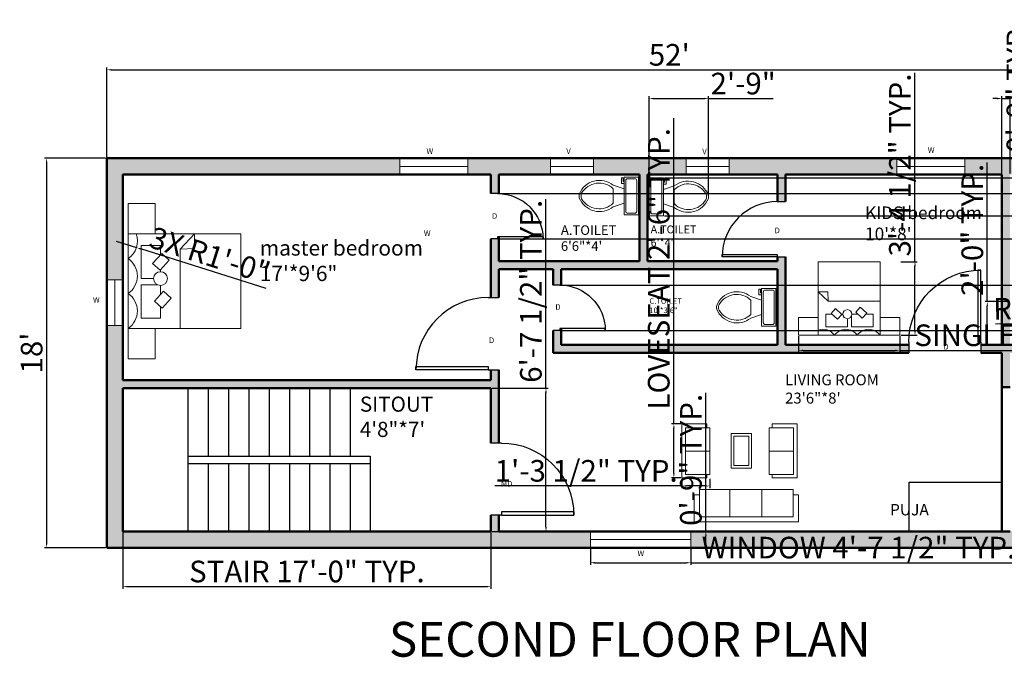
# Model space of a CAD drawing. Units: inches. Extents: x 2225 to 3094, y 1739 to 2599.
# Tile 1 of 5: x 2234 to 2780, y 1739 to 2092. Entities that reach past the tile are written whole.
import ezdxf

# ---------------------------------------------------------------- set-up
doc = ezdxf.new("R2010")
doc.units = ezdxf.units.IN
for name, color, linetype, lineweight in [('A-ANNO-DIMS', 2, 'Continuous', 18), ('A-ANNO-TEXT', 7, 'Continuous', 18), ('A-ANNO-TITL', 7, 'Continuous', 35), ('A-AREA-IDEN', 7, 'Continuous', 18), ('A-DOOR', 4, 'Continuous', 25), ('A-FLOR-CASE', 9, 'Continuous', 25), ('A-FLOR-FIXT', 9, 'Continuous', 18), ('A-FLOR-STRS', 7, 'Continuous', 25), ('A-FURN', 8, 'Continuous', 18), ('A-WALL-PATT', 160, 'Continuous', 13), ('WALL', 7, 'Continuous', 50), ('WINDOW', 130, 'Continuous', 18)]:
    doc.layers.add(name, color=color, linetype=linetype, lineweight=lineweight)
doc.styles.get("Standard").update_dxf_attribs({"font": 'arial.ttf'})
doc.dimstyles.new('ISO-25', dxfattribs={"dimtxt": 12, "dimasz": 2.5, "dimexe": 1.25, "dimexo": 0.625, "dimtad": 1, "dimdec": 0, "dimlunit": 4, "dimtxsty": 'Standard', "dimcen": 2.5, "dimadec": 0, "dimazin": 0, "dimtfac": 1, "dimtdec": 0, "dimtmove": 0, "dimatfit": 3, "dimfxl": 1, "dimarcsym": 0})

# ---------------------------------------------------------------- blocks, each defined once
blk = doc.blocks.new('*U2')
for p, q in [((9.5, -6), (9.5, -2)), ((-10, -8.5), (-8, -8.5)), ((-10, -9.5), (-10, -8.5)), ((-7, -9.5), (-10, -9.5)), ((-8, -8.5), (-8, -8)), ((-7, -8), (-7, -9.5)), ((-4, -8), (-6, -14)), ((4, -8), (6, -14)), ((4, -14), (-4, -14))]:
    blk.add_line(p, q)
blk.add_lwpolyline([(10.5, -8), (10.5, 0), (-10.5, 0), (-10.5, -8)], close=True)
for points in [[(-9.5, -2), (-9.5, -6)], [(8.5, -1), (-8.5, -1)], [(-8.5, -7), (8.5, -7)]]:
    blk.add_lwpolyline(points)
for centre, radius, start, end in [((-8.62, -1.88), 0.884, 81.8699, 188.1301), ((8.62, -1.88), 0.884, 351.8699, 98.1301), ((-8.62, -6.12), 0.884, 171.8699, 278.1301), ((8.62, -6.12), 0.884, 261.8699, 8.1301), ((3.52, -21.58), 12.17, 141.4691, 247.9714), ((4.2, -21.82), 11.33, 136.3677, 238.9468), ((-3.52, -21.58), 12.17, 292.0284, 38.5307), ((-4.2, -21.82), 11.33, 301.053, 43.6321), ((0, -27.88), 4, 245.7318, 294.2682), ((0, -29), 4, 254.8605, 285.1395)]:
    blk.add_arc(centre, radius, start, end)
blk = doc.blocks.new('*U4')
for p, q in [((0, 0), (0, -6)), ((40, 0), (40, -6))]:
    blk.add_line(p, q)
blk.add_lwpolyline([(0, 0), (0, 40), (1.75, 40), (1.75, 0)], close=True)
blk.add_arc((0, 0), 40, 0, 90)
blk = doc.blocks.new('*D7')
at = {"layer": 'A-ANNO-DIMS', "color": 0, "lineweight": -2, "transparency": 16777216}
for p, q in [((2282.56, 2016.04), (2282.56, 2065.75)), ((2285.06, 2064.5), (2904.06, 2064.5)), ((2906.56, 2016.04), (2906.56, 2065.75))]:
    blk.add_line(p, q, dxfattribs=at)
at = {"layer": 'A-ANNO-DIMS', "color": 0, "transparency": 16777216}
for points in [[(2285.06, 2064.92), (2285.06, 2064.08), (2282.56, 2064.5)], [(2904.06, 2064.92), (2904.06, 2064.08), (2906.56, 2064.5)]]:
    blk.add_solid(points, dxfattribs=at)
at = {"layer": 'Defpoints', "color": 0, "transparency": 16777216}
for p in [(2906.56, 2064.5), (2282.56, 2015.41), (2906.56, 2015.41)]:
    blk.add_point(p, dxfattribs=at)
at = {"layer": 'A-ANNO-DIMS', "color": 0, "transparency": 16777216, "insert": (2594.56, 2071.25), "char_height": 12, "attachment_point": 5}
blk.add_mtext("52'", dxfattribs=at)
blk = doc.blocks.new('*D8')
at = {"layer": 'A-ANNO-DIMS', "color": 0, "lineweight": -2, "transparency": 16777216}
for p, q in [((2281.93, 2015.41), (2247.95, 2015.41)), ((2249.2, 2012.91), (2249.2, 1801.91)), ((2281.93, 1799.41), (2247.95, 1799.41))]:
    blk.add_line(p, q, dxfattribs=at)
at = {"layer": 'A-ANNO-DIMS', "color": 0, "transparency": 16777216}
for points in [[(2248.78, 2012.91), (2249.61, 2012.91), (2249.2, 2015.41)], [(2248.78, 1801.91), (2249.61, 1801.91), (2249.2, 1799.41)]]:
    blk.add_solid(points, dxfattribs=at)
at = {"layer": 'Defpoints', "color": 0, "transparency": 16777216}
for p in [(2282.56, 2015.41), (2249.2, 1799.41), (2282.56, 1799.41)]:
    blk.add_point(p, dxfattribs=at)
at = {"layer": 'A-ANNO-DIMS', "color": 0, "transparency": 16777216, "insert": (2242.45, 1907.41), "char_height": 12, "attachment_point": 5, "rotation": 90}
blk.add_mtext("18'", dxfattribs=at)
blk = doc.blocks.new('STAIR-RETURN')
for p, q in [((0, 79.5), (36, 79.5)), ((36, 79.5), (36, 0)), ((47.27, 79.5), (47.27, 41.75)), ((58.52, 79.5), (58.52, 41.75)), ((69.77, 79.5), (69.77, 41.75)), ((81.01, 79.5), (81.01, 41.75)), ((92.26, 79.5), (92.26, 41.75)), ((103.51, 79.5), (103.51, 41.75)), ((114.75, 79.5), (114.75, 41.75)), ((204, 79.5), (126, 79.5)), ((126, 79.5), (126, 41.75)), ((36, 41.75), (126, 41.75)), ((126, 41.75), (137, 41.75)), ((137, 41.75), (137, 0)), ((36, 37.75), (126, 37.75)), ((47.27, 37.75), (47.27, 0)), ((58.52, 37.75), (58.52, 0)), ((69.77, 37.75), (69.77, 0)), ((81.01, 37.75), (81.01, 0)), ((92.26, 37.75), (92.26, 0)), ((103.51, 37.75), (103.51, 0)), ((114.75, 37.75), (114.75, 0)), ((126, 37.75), (137, 37.75)), ((126, 37.75), (126, 0))]:
    blk.add_line(p, q)
blk = doc.blocks.new('BED-MASTER')
for p, q in [((28.8, 60.76), (36.78, 69.23)), ((36.78, 69.23), (36.78, 61.09)), ((36.78, 61.09), (28.8, 60.76)), ((28.8, 16.79), (28.8, 60.76))]:
    blk.add_line(p, q)
for points in [[(0, 69.23), (14.9, 69.23), (14.9, 86.02), (0, 86.02)], [(0, 16.79), (62.39, 16.79), (62.39, 69.23), (0, 69.23)], [(13.53, 52.86), (18.54, 58.39), (22.68, 54.63), (17.67, 49.11)], [(14.58, 31.86), (19.59, 37.39), (23.73, 33.63), (18.72, 28.11)], [(0, 0), (14.9, 0), (14.9, 16.79), (0, 16.79)]]:
    blk.add_lwpolyline(points, close=True)
for points in [[(17.87, 57.65), (17.87, 62.86), (7.1, 62.86), (7.1, 44.44), (14.04, 44.44)], [(17.87, 48.27), (17.87, 49.33)], [(16.36, 40.92), (7.1, 40.92), (7.1, 22.51), (17.87, 22.51), (17.87, 28.87)], [(17.87, 35.5), (17.87, 40.61)]]:
    blk.add_lwpolyline(points)
blk.add_circle((17.87, 44.44), 3.83)
for centre, end in [((-6.76, 65.2), 19.9878), ((-6.76, 45.83), 55.0719), ((-6.76, 26.47), 55.0719)]:
    blk.add_arc(centre, 11.81, 304.9281, end)
blk = doc.blocks.new('BED-SINGLE')
for p, q in [((16.5, 18.81), (10.96, 24.02)), ((10.96, 24.02), (16.28, 24.02)), ((16.28, 24.02), (16.5, 18.81)), ((45.21, 18.81), (16.5, 18.81))]:
    blk.add_line(p, q)
for points in [[(45.21, 0), (45.21, 40.75), (10.96, 40.75), (10.96, 0)], [(21.65, 8.84), (18.05, 12.11), (20.5, 14.81), (24.1, 11.54)], [(35.37, 9.52), (31.76, 12.79), (34.21, 15.49), (37.82, 12.22)], [(10.96, 0), (10.96, 9.73), (0, 9.73), (0, 0)], [(56.18, 0), (56.18, 9.73), (45.21, 9.73), (45.21, 0)]]:
    blk.add_lwpolyline(points, close=True)
for points in [[(18.53, 11.67), (15.12, 11.67), (15.12, 4.64), (27.15, 4.64), (27.15, 9.17)], [(24.65, 11.67), (23.96, 11.67)], [(29.45, 10.68), (29.45, 4.64), (41.48, 4.64), (41.48, 11.67), (37.32, 11.67)], [(32.99, 11.67), (29.65, 11.67)]]:
    blk.add_lwpolyline(points)
blk.add_circle((27.15, 11.67), 2.5)
for centre, end in [((13.6, -4.42), 109.9878), ((26.25, -4.42), 145.0719), ((38.89, -4.42), 145.0719)]:
    blk.add_arc(centre, 7.71, 34.9281, end)
blk = doc.blocks.new('SOFA-THREE-SEAT')
for p, q in [((19.92, 17.92), (19.92, 2.75)), ((37.66, 17.92), (37.66, 2.75)), ((3.02, 14.97), (0, 14.97)), ((0, 14.97), (0, 0)), ((57.91, 14.97), (54.99, 14.97)), ((57.91, 0), (57.91, 14.97)), ((0, 0), (57.91, 0))]:
    blk.add_line(p, q)
blk.add_lwpolyline([(3.02, 2.75), (54.99, 2.75), (54.99, 17.92), (3.02, 17.92)], close=True)
blk = doc.blocks.new('SOFA-TWO-SEAT')
for p, q in [((1.66, 27.74), (1.66, 29.95)), ((1.66, 29.95), (15.43, 29.95)), ((15.43, 29.95), (15.43, 0)), ((0, 14.84), (13.39, 14.84)), ((1.66, 0), (1.66, 1.94)), ((15.43, 0), (1.66, 0))]:
    blk.add_line(p, q)
blk.add_lwpolyline([(13.39, 1.94), (0, 1.94), (0, 27.74), (13.39, 27.74)], close=True)
blk = doc.blocks.new('TABLE-COFFEE')
for points in [[(0, 0), (11.17, 0), (11.17, 19.11), (0, 19.11)], [(1.5, 1.5), (9.67, 1.5), (9.67, 17.61), (1.5, 17.61)]]:
    blk.add_lwpolyline(points, close=True)
blk = doc.blocks.new('WIN-55P7IN')
blk.add_line((0, 4.5), (55.68, 4.5))
blk.add_lwpolyline([(0, 0), (55.68, 0), (55.68, 9), (0, 9)], close=True)
blk = doc.blocks.new('*D26')
at = {"layer": 'A-ANNO-DIMS', "color": 0, "lineweight": -2, "transparency": 16777216}
for p, q in [((2666.23, 1916.66), (2666.23, 1907.61)), ((2722.41, 1916.66), (2722.41, 1907.61)), ((2668.73, 1908.86), (2719.91, 1908.86)), ((2722.41, 1908.86), (2904.52, 1908.86))]:
    blk.add_line(p, q, dxfattribs=at)
at = {"layer": 'A-ANNO-DIMS', "color": 0, "transparency": 16777216}
for points in [[(2668.73, 1909.27), (2668.73, 1908.44), (2666.23, 1908.86)], [(2719.91, 1909.27), (2719.91, 1908.44), (2722.41, 1908.86)]]:
    blk.add_solid(points, dxfattribs=at)
at = {"layer": 'Defpoints', "color": 0, "transparency": 16777216}
for p in [(2666.23, 1917.28), (2722.41, 1917.28), (2722.41, 1908.86)]:
    blk.add_point(p, dxfattribs=at)
at = {"layer": 'A-ANNO-DIMS', "color": 0, "transparency": 16777216, "insert": (2814.71, 1915.69), "char_height": 12, "attachment_point": 5}
blk.add_mtext('SINGLE BED 4\'-8" TYP.', dxfattribs=at)
blk = doc.blocks.new('*D27')
at = {"layer": 'A-ANNO-DIMS', "color": 0, "lineweight": -2, "transparency": 16777216}
for p, q in [((2730.83, 1958.03), (2730.83, 2062.88)), ((2723.03, 1958.03), (2732.08, 1958.03)), ((2730.83, 1919.78), (2730.83, 1955.53)), ((2723.03, 1917.28), (2732.08, 1917.28))]:
    blk.add_line(p, q, dxfattribs=at)
at = {"layer": 'A-ANNO-DIMS', "color": 0, "transparency": 16777216}
for points in [[(2730.42, 1955.53), (2731.25, 1955.53), (2730.83, 1958.03)], [(2730.42, 1919.78), (2731.25, 1919.78), (2730.83, 1917.28)]]:
    blk.add_solid(points, dxfattribs=at)
at = {"layer": 'Defpoints', "color": 0, "transparency": 16777216}
for p in [(2722.41, 1958.03), (2730.83, 1958.03), (2722.41, 1917.28)]:
    blk.add_point(p, dxfattribs=at)
at = {"layer": 'A-ANNO-DIMS', "color": 0, "transparency": 16777216, "insert": (2724, 2011.7), "char_height": 12, "attachment_point": 5, "rotation": 90}
blk.add_mtext('3\'-4 1/2" TYP.', dxfattribs=at)
blk = doc.blocks.new('*D34')
at = {"layer": 'A-ANNO-DIMS', "color": 0, "lineweight": -2, "transparency": 16777216}
for p, q in [((2597.09, 1868.1), (2597.09, 2037.63)), ((2600.96, 1868.1), (2595.84, 1868.1)), ((2597.09, 1840.65), (2597.09, 1865.6)), ((2600.96, 1838.15), (2595.84, 1838.15))]:
    blk.add_line(p, q, dxfattribs=at)
at = {"layer": 'A-ANNO-DIMS', "color": 0, "transparency": 16777216}
for points in [[(2596.67, 1865.6), (2597.51, 1865.6), (2597.09, 1868.1)], [(2596.67, 1840.65), (2597.51, 1840.65), (2597.09, 1838.15)]]:
    blk.add_solid(points, dxfattribs=at)
at = {"layer": 'Defpoints', "color": 0, "transparency": 16777216}
for p in [(2597.09, 1868.1), (2601.58, 1868.1), (2601.58, 1838.15)]:
    blk.add_point(p, dxfattribs=at)
at = {"layer": 'A-ANNO-DIMS', "color": 0, "transparency": 16777216, "insert": (2590.26, 1954.11), "char_height": 12, "attachment_point": 5, "rotation": 90}
blk.add_mtext('LOVESEAT 2\'-6" TYP.', dxfattribs=at)
blk = doc.blocks.new('*D35')
at = {"layer": 'A-ANNO-DIMS', "color": 0, "lineweight": -2, "transparency": 16777216}
for p, q in [((2601.58, 1837.52), (2601.58, 1832.41)), ((2617.01, 1837.52), (2617.01, 1832.41)), ((2601.58, 1833.66), (2497.86, 1833.66)), ((2614.51, 1833.66), (2604.08, 1833.66))]:
    blk.add_line(p, q, dxfattribs=at)
at = {"layer": 'A-ANNO-DIMS', "color": 0, "transparency": 16777216}
for points in [[(2604.08, 1834.07), (2604.08, 1833.24), (2601.58, 1833.66)], [(2614.51, 1834.07), (2614.51, 1833.24), (2617.01, 1833.66)]]:
    blk.add_solid(points, dxfattribs=at)
at = {"layer": 'Defpoints', "color": 0, "transparency": 16777216}
for p in [(2601.58, 1838.15), (2617.01, 1838.15), (2601.58, 1833.66)]:
    blk.add_point(p, dxfattribs=at)
at = {"layer": 'A-ANNO-DIMS', "color": 0, "transparency": 16777216, "insert": (2548.47, 1840.49), "char_height": 12, "attachment_point": 5}
blk.add_mtext('1\'-3 1/2" TYP.', dxfattribs=at)
blk = doc.blocks.new('*D43')
at = {"layer": 'A-ANNO-DIMS', "color": 0, "lineweight": -2, "transparency": 16777216}
for p, q in [((2770.92, 1935.91), (2770.92, 2013.01)), ((2782.93, 1935.91), (2769.67, 1935.91)), ((2770.92, 1914.41), (2770.92, 1933.41)), ((2782.93, 1911.91), (2769.67, 1911.91))]:
    blk.add_line(p, q, dxfattribs=at)
at = {"layer": 'A-ANNO-DIMS', "color": 0, "transparency": 16777216}
for points in [[(2770.5, 1933.41), (2771.34, 1933.41), (2770.92, 1935.91)], [(2770.5, 1914.41), (2771.34, 1914.41), (2770.92, 1911.91)]]:
    blk.add_solid(points, dxfattribs=at)
at = {"layer": 'Defpoints', "color": 0, "transparency": 16777216}
for p in [(2770.92, 1935.91), (2783.56, 1935.91), (2783.56, 1911.91)]:
    blk.add_point(p, dxfattribs=at)
at = {"layer": 'A-ANNO-DIMS', "color": 0, "transparency": 16777216, "insert": (2764.17, 1975.71), "char_height": 12, "attachment_point": 5, "rotation": 90}
blk.add_mtext('2\'-0" TYP.', dxfattribs=at)
blk = doc.blocks.new('*D44')
at = {"layer": 'A-ANNO-DIMS', "color": 0, "lineweight": -2, "transparency": 16777216}
for p, q in [((2291.56, 1807.79), (2291.56, 1776.56)), ((2495.56, 1807.79), (2495.56, 1776.56)), ((2294.06, 1777.81), (2493.06, 1777.81))]:
    blk.add_line(p, q, dxfattribs=at)
at = {"layer": 'A-ANNO-DIMS', "color": 0, "transparency": 16777216}
for points in [[(2294.06, 1778.23), (2294.06, 1777.39), (2291.56, 1777.81)], [(2493.06, 1778.23), (2493.06, 1777.39), (2495.56, 1777.81)]]:
    blk.add_solid(points, dxfattribs=at)
at = {"layer": 'Defpoints', "color": 0, "transparency": 16777216}
for p in [(2291.56, 1808.41), (2495.56, 1808.41), (2495.56, 1777.81)]:
    blk.add_point(p, dxfattribs=at)
at = {"layer": 'A-ANNO-DIMS', "color": 0, "transparency": 16777216, "insert": (2393.56, 1784.64), "char_height": 12, "attachment_point": 5}
blk.add_mtext('STAIR 17\'-0" TYP.', dxfattribs=at)
blk = doc.blocks.new('*D45')
at = {"layer": 'A-ANNO-DIMS', "color": 0, "lineweight": -2, "transparency": 16777216}
for p, q in [((2526.16, 1887.91), (2526.16, 1992.83)), ((2496.18, 1887.91), (2527.41, 1887.91)), ((2526.16, 1810.91), (2526.16, 1885.41)), ((2496.18, 1808.41), (2527.41, 1808.41))]:
    blk.add_line(p, q, dxfattribs=at)
at = {"layer": 'A-ANNO-DIMS', "color": 0, "transparency": 16777216}
for points in [[(2525.74, 1885.41), (2526.57, 1885.41), (2526.16, 1887.91)], [(2525.74, 1810.91), (2526.57, 1810.91), (2526.16, 1808.41)]]:
    blk.add_solid(points, dxfattribs=at)
at = {"layer": 'Defpoints', "color": 0, "transparency": 16777216}
for p in [(2495.56, 1887.91), (2526.16, 1887.91), (2495.56, 1808.41)]:
    blk.add_point(p, dxfattribs=at)
at = {"layer": 'A-ANNO-DIMS', "color": 0, "transparency": 16777216, "insert": (2519.33, 1941.62), "char_height": 12, "attachment_point": 5, "rotation": 90}
blk.add_mtext('6\'-7 1/2" TYP.', dxfattribs=at)
blk = doc.blocks.new('*D47')
at = {"layer": 'A-ANNO-DIMS', "color": 0, "lineweight": -2, "transparency": 16777216}
for p, q in [((2795.9, 2015.41), (2795.9, 2092.31)), ((2800.91, 2015.41), (2794.65, 2015.41)), ((2795.9, 2008.91), (2795.9, 2012.91)), ((2800.91, 2006.41), (2794.65, 2006.41))]:
    blk.add_line(p, q, dxfattribs=at)
at = {"layer": 'A-ANNO-DIMS', "color": 0, "transparency": 16777216}
for points in [[(2795.48, 2012.91), (2796.32, 2012.91), (2795.9, 2015.41)], [(2795.48, 2008.91), (2796.32, 2008.91), (2795.9, 2006.41)]]:
    blk.add_solid(points, dxfattribs=at)
at = {"layer": 'Defpoints', "color": 0, "transparency": 16777216}
for p in [(2795.9, 2015.41), (2801.54, 2015.41), (2801.54, 2006.41)]:
    blk.add_point(p, dxfattribs=at)
at = {"layer": 'A-ANNO-DIMS', "color": 0, "transparency": 16777216, "insert": (2789.15, 2055.11), "char_height": 12, "attachment_point": 5, "rotation": 90}
blk.add_mtext('0\'-9" TYP.', dxfattribs=at)
blk = doc.blocks.new('*D52')
at = {"layer": 'A-ANNO-DIMS', "color": 0, "lineweight": -2, "transparency": 16777216}
for p, q in [((2550.8, 1798.79), (2550.8, 1789.81)), ((2606.48, 1798.79), (2606.48, 1789.81)), ((2553.3, 1791.06), (2603.98, 1791.06)), ((2606.48, 1791.06), (2790.04, 1791.06))]:
    blk.add_line(p, q, dxfattribs=at)
at = {"layer": 'A-ANNO-DIMS', "color": 0, "transparency": 16777216}
for points in [[(2553.3, 1791.48), (2553.3, 1790.64), (2550.8, 1791.06)], [(2603.98, 1791.48), (2603.98, 1790.64), (2606.48, 1791.06)]]:
    blk.add_solid(points, dxfattribs=at)
at = {"layer": 'Defpoints', "color": 0, "transparency": 16777216}
for p in [(2550.8, 1799.41), (2606.48, 1799.41), (2606.48, 1791.06)]:
    blk.add_point(p, dxfattribs=at)
at = {"layer": 'A-ANNO-DIMS', "color": 0, "transparency": 16777216, "insert": (2699.51, 1797.89), "char_height": 12, "attachment_point": 5}
blk.add_mtext('WINDOW 4\'-7 1/2" TYP.', dxfattribs=at)
blk = doc.blocks.new('*D53')
at = {"layer": 'A-ANNO-DIMS', "color": 0, "lineweight": -2, "transparency": 16777216}
for p, q in [((2614.83, 1808.41), (2614.83, 1885.31)), ((2607.11, 1808.41), (2616.08, 1808.41)), ((2614.83, 1801.91), (2614.83, 1805.91)), ((2607.11, 1799.41), (2616.08, 1799.41))]:
    blk.add_line(p, q, dxfattribs=at)
at = {"layer": 'A-ANNO-DIMS', "color": 0, "transparency": 16777216}
for points in [[(2614.42, 1805.91), (2615.25, 1805.91), (2614.83, 1808.41)], [(2614.42, 1801.91), (2615.25, 1801.91), (2614.83, 1799.41)]]:
    blk.add_solid(points, dxfattribs=at)
at = {"layer": 'Defpoints', "color": 0, "transparency": 16777216}
for p in [(2606.48, 1808.41), (2614.83, 1808.41), (2606.48, 1799.41)]:
    blk.add_point(p, dxfattribs=at)
at = {"layer": 'A-ANNO-DIMS', "color": 0, "transparency": 16777216, "insert": (2608.08, 1848.11), "char_height": 12, "attachment_point": 5, "rotation": 90}
blk.add_mtext('0\'-9" TYP.', dxfattribs=at)
blk = doc.blocks.new('*D71')
at = {"layer": 'A-ANNO-DIMS', "color": 0, "lineweight": -2, "transparency": 16777216}
for p, q in [((2939.71, 1995.85), (2939.71, 2031.7)), ((2500.68, 1995.85), (2940.96, 1995.85)), ((2939.71, 1973.17), (2939.71, 1993.35)), ((2499.96, 1970.67), (2940.96, 1970.67))]:
    blk.add_line(p, q, dxfattribs=at)
at = {"layer": 'A-ANNO-DIMS', "color": 0, "transparency": 16777216}
for points in [[(2939.29, 1993.35), (2940.12, 1993.35), (2939.71, 1995.85)], [(2939.29, 1973.17), (2940.12, 1973.17), (2939.71, 1970.67)]]:
    blk.add_solid(points, dxfattribs=at)
at = {"layer": 'Defpoints', "color": 0, "transparency": 16777216}
for p in [(2500.06, 1995.85), (2939.71, 1995.85), (2499.34, 1970.67)]:
    blk.add_point(p, dxfattribs=at)
at = {"layer": 'A-ANNO-DIMS', "color": 0, "transparency": 16777216, "insert": (2933.06, 2015.03), "char_height": 12, "attachment_point": 5, "rotation": 90}
blk.add_mtext('2\'-1"', dxfattribs=at)
blk = doc.blocks.new('*D73')
at = {"layer": 'A-ANNO-DIMS', "color": 0, "lineweight": -2, "transparency": 16777216}
for p, q in [((2939.71, 1945.09), (2939.71, 1980.94)), ((2535.18, 1945.09), (2940.96, 1945.09)), ((2939.71, 1922.41), (2939.71, 1942.59)), ((2534.46, 1919.91), (2940.96, 1919.91))]:
    blk.add_line(p, q, dxfattribs=at)
at = {"layer": 'A-ANNO-DIMS', "color": 0, "transparency": 16777216}
for points in [[(2939.29, 1942.59), (2940.12, 1942.59), (2939.71, 1945.09)], [(2939.29, 1922.41), (2940.12, 1922.41), (2939.71, 1919.91)]]:
    blk.add_solid(points, dxfattribs=at)
at = {"layer": 'Defpoints', "color": 0, "transparency": 16777216}
for p in [(2534.56, 1945.09), (2939.71, 1945.09), (2533.84, 1919.91)]:
    blk.add_point(p, dxfattribs=at)
at = {"layer": 'A-ANNO-DIMS', "color": 0, "transparency": 16777216, "insert": (2933.06, 1964.27), "char_height": 12, "attachment_point": 5, "rotation": 90}
blk.add_mtext('2\'-1"', dxfattribs=at)
blk = doc.blocks.new('*D76')
at = {"layer": 'A-ANNO-DIMS', "color": 0, "lineweight": -2, "transparency": 16777216}
for p, q in [((2583.35, 2005.22), (2583.35, 2049.81)), ((2585.85, 2048.56), (2613.85, 2048.56)), ((2616.35, 1994.72), (2616.35, 2049.81)), ((2616.35, 2048.56), (2652.2, 2048.56))]:
    blk.add_line(p, q, dxfattribs=at)
at = {"layer": 'A-ANNO-DIMS', "color": 0, "transparency": 16777216}
for points in [[(2585.85, 2048.98), (2585.85, 2048.14), (2583.35, 2048.56)], [(2613.85, 2048.98), (2613.85, 2048.14), (2616.35, 2048.56)]]:
    blk.add_solid(points, dxfattribs=at)
at = {"layer": 'Defpoints', "color": 0, "transparency": 16777216}
for p in [(2616.35, 2048.56), (2583.35, 2004.59), (2616.35, 1994.09)]:
    blk.add_point(p, dxfattribs=at)
at = {"layer": 'A-ANNO-DIMS', "color": 0, "transparency": 16777216, "insert": (2635.53, 2055.31), "char_height": 12, "attachment_point": 5}
blk.add_mtext('2\'-9"', dxfattribs=at)
blk = doc.blocks.new('*D77')
at = {"layer": 'A-ANNO-DIMS', "color": 0, "lineweight": -2, "transparency": 16777216}
for p, q in [((2939.71, 2004.59), (2939.71, 2039.11)), ((2591.98, 2004.59), (2940.96, 2004.59)), ((2939.71, 1986.09), (2939.71, 2002.09)), ((2591.98, 1983.59), (2940.96, 1983.59))]:
    blk.add_line(p, q, dxfattribs=at)
at = {"layer": 'A-ANNO-DIMS', "color": 0, "transparency": 16777216}
for points in [[(2939.29, 2002.09), (2940.12, 2002.09), (2939.71, 2004.59)], [(2939.29, 1986.09), (2940.12, 1986.09), (2939.71, 1983.59)]]:
    blk.add_solid(points, dxfattribs=at)
at = {"layer": 'Defpoints', "color": 0, "transparency": 16777216}
for p in [(2591.35, 2004.59), (2939.71, 2004.59), (2591.35, 1983.59)]:
    blk.add_point(p, dxfattribs=at)
at = {"layer": 'A-ANNO-DIMS', "color": 0, "transparency": 16777216, "insert": (2932.96, 2023.1), "char_height": 12, "attachment_point": 5, "rotation": 90}
blk.add_mtext('1\'-9"', dxfattribs=at)
blk = doc.blocks.new('*D78')
at = {"layer": 'A-ANNO-DIMS', "color": 0, "lineweight": -2, "transparency": 16777216}
for p, q in [((2776.56, 2048.56), (2774.06, 2048.56)), ((2779.06, 2007.04), (2779.06, 2049.81)), ((2779.06, 2048.56), (2783.56, 2048.56)), ((2783.56, 2007.04), (2783.56, 2049.81)), ((2786.06, 2048.56), (2849.67, 2048.56))]:
    blk.add_line(p, q, dxfattribs=at)
at = {"layer": 'A-ANNO-DIMS', "color": 0, "transparency": 16777216}
for points in [[(2776.56, 2048.98), (2776.56, 2048.14), (2779.06, 2048.56)], [(2786.06, 2048.98), (2786.06, 2048.14), (2783.56, 2048.56)]]:
    blk.add_solid(points, dxfattribs=at)
at = {"layer": 'Defpoints', "color": 0, "transparency": 16777216}
for p in [(2783.56, 2048.56), (2779.06, 2006.41), (2783.56, 2006.41)]:
    blk.add_point(p, dxfattribs=at)
at = {"layer": 'A-ANNO-DIMS', "color": 0, "transparency": 16777216, "insert": (2819.11, 2055.39), "char_height": 12, "attachment_point": 5}
blk.add_mtext('0\'-4 1/2"', dxfattribs=at)
blk = doc.blocks.new('*D79')
at = {"layer": 'A-ANNO-DIMS', "color": 0, "lineweight": -2, "transparency": 16777216}
for p, q in [((2775.41, 1923.56), (2850.49, 1924.61)), ((2877.38, 1924.99), (2852.99, 1924.65))]:
    blk.add_line(p, q, dxfattribs=at)
at = {"layer": 'A-ANNO-DIMS', "color": 0, "transparency": 16777216}
blk.add_solid([(2850.49, 1925.03), (2850.5, 1924.2), (2852.99, 1924.65)], dxfattribs=at)
at = {"layer": 'Defpoints', "color": 0, "transparency": 16777216}
for p in [(2852.99, 1924.65), (2877.38, 1924.99)]:
    blk.add_point(p, dxfattribs=at)
at = {"layer": 'A-ANNO-DIMS', "color": 0, "transparency": 16777216, "insert": (2811.6, 1930.9), "char_height": 12, "attachment_point": 5, "rotation": 0.8061}
blk.add_mtext('R2\'-0 1/2"', dxfattribs=at)
blk = doc.blocks.new('*D80')
at = {"layer": 'A-ANNO-DIMS', "color": 0, "lineweight": -2, "transparency": 16777216}
for p, q in [((2287.72, 1969.44), (2298.98, 1965.89)), ((2370.89, 1943.16), (2301.37, 1965.13))]:
    blk.add_line(p, q, dxfattribs=at)
at = {"layer": 'A-ANNO-DIMS', "color": 0, "transparency": 16777216}
blk.add_solid([(2301.49, 1965.53), (2301.24, 1964.74), (2298.98, 1965.89)], dxfattribs=at)
at = {"layer": 'Defpoints', "color": 0, "transparency": 16777216}
for p in [(2287.72, 1969.44), (2298.98, 1965.89)]:
    blk.add_point(p, dxfattribs=at)
at = {"layer": 'A-ANNO-DIMS', "color": 0, "transparency": 16777216, "insert": (2339.35, 1960.21), "char_height": 12, "attachment_point": 5, "rotation": 342.4603}
blk.add_mtext('3X R1\'-0"', dxfattribs=at)

msp = doc.modelspace()

# ---------------------------------------------------------------- hatches: boundary and pattern name
at = {"layer": 'A-WALL-PATT'}
h = msp.add_hatch(color=256, dxfattribs=at)
h.dxf.hatch_style = 1
h.paths.add_polyline_path([(2445.16, 2015.41), (2282.56, 2015.41), (2282.56, 1948.06), (2291.56, 1948.06), (2291.56, 2006.41), (2445.16, 2006.41)], flags=17)
h.paths.add_polyline_path([(2528.69, 2015.41), (2482.76, 2015.41), (2482.76, 2006.41), (2495.56, 2006.41), (2495.56, 1995.86), (2499.34, 1995.86, -0.007163), (2500.06, 1995.85), (2500.06, 2006.41), (2528.69, 2006.41)], flags=17)
h.paths.add_polyline_path([(2867.81, 1911.91), (2783.56, 1911.91), (2783.56, 1935.91), (2783.56, 2006.41), (2801.54, 2006.41), (2801.54, 2015.41), (2758.39, 2015.41), (2758.39, 2006.41), (2779.06, 2006.41), (2779.06, 1911.91), (2767.43, 1911.91), (2767.43, 1907.41), (2779.06, 1907.41), (2779.06, 1888.45), (2783.56, 1888.45), (2783.56, 1907.41), (2867.81, 1907.41)])
h.paths.add_polyline_path([(2906.56, 2015.41), (2839.14, 2015.41), (2839.14, 2006.41), (2897.56, 2006.41), (2897.56, 1911.91), (2897.56, 1907.41), (2897.56, 1845.22), (2906.56, 1845.22)])
h.paths.add_polyline_path([(2906.56, 1817.4), (2897.56, 1817.4), (2897.56, 1808.41), (2860.08, 1808.41), (2860.08, 1799.41), (2906.56, 1799.41)])
h.paths.add_polyline_path([(2815.14, 1808.41), (2783.56, 1808.41), (2779.06, 1808.41), (2727.64, 1808.41), (2606.48, 1808.41), (2606.48, 1799.41), (2815.14, 1799.41)])
h.paths.add_polyline_path([(2780.45, 1854.18), (2785.35, 1854.18), (2785.35, 1860.55), (2780.45, 1860.55)], flags=9)
h.paths.add_polyline_path([(2500.16, 1831.65), (2508.42, 1831.65), (2508.42, 1838.02), (2500.16, 1838.02)], flags=25)
h.paths.add_polyline_path([(2745.49, 1907.67), (2750.15, 1907.67), (2750.15, 1914.04), (2745.49, 1914.04)], flags=9)
h.paths.add_polyline_path([(2651.86, 1972.18), (2656.53, 1972.18), (2656.53, 1978.54), (2651.86, 1978.54)], flags=9)
h.paths.add_polyline_path([(2493.47, 1911.25), (2498.13, 1911.25), (2498.13, 1917.61), (2493.47, 1917.61)], flags=25)
h.paths.add_polyline_path([(2530.27, 1929.7), (2534.93, 1929.7), (2534.93, 1936.07), (2530.27, 1936.07)], flags=25)
h.paths.add_polyline_path([(2432.89, 1863.65), (2450.26, 1863.65), (2450.26, 1875.18), (2432.89, 1875.18)], flags=25)
h.paths.add_polyline_path([(2735.79, 1821.76), (2748.37, 1821.76), (2748.37, 1828.13), (2735.79, 1828.13)], flags=9)
h.paths.add_polyline_path([(2717.02, 1870.02), (2747.35, 1870.02), (2747.35, 1881.55), (2717.02, 1881.55)], flags=9)
h.paths.add_polyline_path([(2839.5, 1851.69), (2856.29, 1851.69), (2856.29, 1863.22), (2839.5, 1863.22)], flags=25)
h.paths.add_polyline_path([(2825.64, 1966.59), (2846.28, 1966.59), (2846.28, 1978.12), (2825.64, 1978.12)], flags=25)
h.paths.add_polyline_path([(2692.05, 1977.43), (2722.05, 1977.43), (2722.05, 1988.96), (2692.05, 1988.96)], flags=9)
h.paths.add_polyline_path([(2282.56, 1948.06), (2291.56, 1948.06), (2291.56, 2006.41), (2445.16, 2006.41), (2445.16, 2015.41), (2282.56, 2015.41)])
h.paths.add_polyline_path([(2291.56, 1922.71), (2282.56, 1922.71), (2282.56, 1799.41), (2550.8, 1799.41), (2550.8, 1808.41), (2500.06, 1808.41), (2500.06, 1817.48), (2495.56, 1817.48), (2495.56, 1808.41), (2291.56, 1808.41), (2291.56, 1887.91), (2327.56, 1887.91), (2495.56, 1887.91), (2495.56, 1857.48), (2500.06, 1857.48), (2500.06, 1887.91), (2500.06, 1898.14), (2495.56, 1898.14), (2495.56, 1892.41), (2291.56, 1892.41)])
h = msp.add_hatch(color=256, dxfattribs=at)
h.dxf.hatch_style = 1
h.paths.add_polyline_path([(2727.43, 1911.91), (2659.06, 1911.91), (2659.06, 1960.76), (2654.56, 1960.76), (2654.56, 1958.41), (2582.56, 1958.41), (2582.56, 2006.41), (2603.88, 2006.41), (2603.88, 2015.41), (2552.55, 2015.41), (2552.55, 2006.41), (2578.06, 2006.41), (2578.06, 1958.41), (2500.06, 1958.41), (2500.06, 1970.67), (2499.34, 1970.67), (2495.56, 1970.67), (2495.56, 1938.14), (2500.06, 1938.14), (2500.06, 1953.91), (2530.06, 1953.91), (2530.06, 1945.1), (2533.84, 1945.1, -0.007163), (2534.56, 1945.09), (2534.56, 1953.91), (2578.06, 1953.91), (2582.56, 1953.91), (2654.56, 1953.91), (2654.56, 1911.91), (2582.56, 1911.91), (2581.71, 1911.91), (2578.06, 1911.91), (2534.56, 1911.91), (2534.56, 1919.91), (2533.84, 1919.91), (2530.06, 1919.91), (2530.06, 1907.41), (2659.06, 1907.41), (2727.43, 1907.41)])
h.paths.add_polyline_path([(2720.79, 2015.41), (2627.74, 2015.41), (2627.74, 2006.41), (2654.56, 2006.41), (2654.56, 1991.37), (2659.06, 1991.37), (2659.06, 2006.41), (2720.79, 2006.41)], flags=17)
h.paths.add_polyline_path([(2445.16, 2015.41), (2282.56, 2015.41), (2282.56, 1948.06), (2291.56, 1948.06), (2291.56, 2006.41), (2445.16, 2006.41)])

# ---------------------------------------------------------------- linework, layer by layer
at = {"layer": 'A-FLOR-CASE'}
msp.add_lwpolyline([(2779.06, 1808.41), (2727.64, 1808.41), (2727.64, 1835.7), (2779.06, 1835.7)], close=True, dxfattribs=at)
at = {"layer": 'WALL'}
for p, q in [((2291.56, 2006.41), (2495.56, 2006.41)), ((2495.56, 2006.41), (2495.56, 1995.86)), ((2500.06, 2006.41), (2500.06, 1995.85)), ((2500.06, 2006.41), (2500.06, 1995.85)), ((2578.06, 2006.41), (2578.06, 1958.41)), ((2582.56, 2006.41), (2582.56, 1958.41)), ((2654.56, 2006.41), (2654.56, 1991.37)), ((2659.06, 2006.41), (2659.06, 1991.37)), ((2779.06, 2006.41), (2779.06, 1911.91)), ((2500.06, 1971.77), (2500.06, 1958.41)), ((2500.06, 1971.77), (2500.06, 1958.41)), ((2495.56, 1970.67), (2495.56, 1938.14)), ((2654.56, 1960.76), (2654.56, 1958.41)), ((2659.06, 1960.76), (2659.06, 1911.91)), ((2500.06, 1958.41), (2578.06, 1958.41)), ((2582.56, 1958.41), (2654.56, 1958.41)), ((2500.06, 1953.91), (2500.06, 1938.14)), ((2500.06, 1953.91), (2530.06, 1953.91)), ((2530.06, 1945.1), (2530.06, 1953.91)), ((2534.56, 1953.91), (2578.06, 1953.91)), ((2534.56, 1945.09), (2534.56, 1953.91)), ((2578.06, 1953.91), (2582.56, 1953.91)), ((2582.56, 1953.91), (2654.56, 1953.91)), ((2654.56, 1953.91), (2654.56, 1911.91)), ((2654.56, 1953.91), (2654.56, 1911.91)), ((2530.06, 1907.41), (2530.06, 1919.91)), ((2534.56, 1911.91), (2534.56, 1921.01)), ((2578.06, 1911.91), (2534.56, 1911.91)), ((2578.06, 1911.91), (2581.71, 1911.91)), ((2581.71, 1911.91), (2584.98, 1911.91)), ((2654.56, 1911.91), (2582.56, 1911.91)), ((2659.06, 1911.91), (2727.43, 1911.91)), ((2767.43, 1911.91), (2779.06, 1911.91)), ((2659.06, 1907.41), (2530.06, 1907.41)), ((2659.06, 1907.41), (2727.43, 1907.41)), ((2767.43, 1907.41), (2779.06, 1907.41)), ((2779.06, 1907.41), (2779.06, 1808.41)), ((2495.56, 1898.14), (2495.56, 1892.41)), ((2500.06, 1898.14), (2500.06, 1887.91)), ((2495.56, 1892.41), (2291.56, 1892.41)), ((2495.56, 1887.91), (2291.56, 1887.91)), ((2495.56, 1887.91), (2495.56, 1857.48)), ((2500.06, 1887.91), (2500.06, 1857.48)), ((2779.06, 1888.45), (2783.56, 1888.45)), ((2495.56, 1817.48), (2495.56, 1808.41)), ((2500.06, 1817.48), (2500.06, 1808.41)), ((2779.06, 1808.41), (2777.56, 1808.41)), ((2779.06, 1808.41), (2783.56, 1808.41))]:
    msp.add_line(p, q, dxfattribs=at)
msp.add_lwpolyline([(2282.56, 1799.41), (2906.56, 1799.41), (2906.56, 2015.41), (2282.56, 2015.41)], close=True, dxfattribs=at)
for points in [[(2495.56, 2006.41), (2291.56, 2006.41), (2291.56, 1892.41)], [(2578.06, 2006.41), (2500.06, 2006.41)], [(2654.56, 2006.41), (2582.56, 2006.41)], [(2779.06, 2006.41), (2659.06, 2006.41)], [(2291.56, 1887.91), (2291.56, 1808.41), (2495.56, 1808.41)], [(2500.06, 1808.41), (2779.06, 1808.41)]]:
    msp.add_lwpolyline(points, dxfattribs=at)
at = {"layer": 'WINDOW'}
for p, q in [((2445.16, 2010.91), (2482.76, 2010.91)), ((2528.69, 2010.91), (2552.55, 2010.91)), ((2603.88, 2010.91), (2627.74, 2010.91)), ((2720.79, 2010.91), (2758.39, 2010.91)), ((2287.06, 1948.06), (2287.06, 1922.71))]:
    msp.add_line(p, q, dxfattribs=at)
for points in [[(2482.76, 2006.41), (2445.16, 2006.41), (2445.16, 2015.41), (2482.76, 2015.41)], [(2528.69, 2006.41), (2552.55, 2006.41), (2552.55, 2015.41), (2528.69, 2015.41)], [(2603.88, 2006.41), (2627.74, 2006.41), (2627.74, 2015.41), (2603.88, 2015.41)], [(2758.39, 2006.41), (2720.79, 2006.41), (2720.79, 2015.41), (2758.39, 2015.41)], [(2282.56, 1948.06), (2291.56, 1948.06), (2291.56, 1922.71), (2282.56, 1922.71)]]:
    msp.add_lwpolyline(points, close=True, dxfattribs=at)

# ---------------------------------------------------------------- block references
at = {"layer": 'A-DOOR'}
for p, xscale, yscale, zscale, rotation in [((2499.34, 1970.67), -0.6297308224195742, 0.6297308224195742, 0.6297308224195742, 270), ((2654.47, 1960.76), 0.7652481811317178, 0.7652481811317178, 0.7652481811317178, 89.99999999999999), ((2533.84, 1919.91), -0.6297308224195742, 0.6297308224195742, 0.6297308224195742, 270)]:
    msp.add_blockref('*U4', p, dxfattribs=dict(at, xscale=xscale, yscale=yscale, zscale=zscale, rotation=rotation))
at = {"layer": 'A-DOOR', "xscale": -1}
msp.add_blockref('*U4', (2767.43, 1913.41), dxfattribs=at)
at = {"layer": 'A-DOOR', "rotation": 89.99999999999999}
msp.add_blockref('*U4', (2494.06, 1898.14), dxfattribs=at)
at = {"layer": 'A-DOOR', "xscale": -1, "rotation": 270}
msp.add_blockref('*U4', (2501.56, 1817.48), dxfattribs=at)
at = {"layer": 'A-FLOR-FIXT', "rotation": 270}
for p in [(2577.48, 1994.51), (2653.71, 1932.75)]:
    msp.add_blockref('*U2', p, dxfattribs=at)
at = {"layer": 'A-FLOR-FIXT', "xscale": -1, "rotation": 90}
msp.add_blockref('*U2', (2583.35, 1994.09), dxfattribs=at)
at = {"layer": 'A-FLOR-STRS'}
msp.add_blockref('STAIR-RETURN', (2291.56, 1808.41), dxfattribs=at)
at = {"layer": 'A-FURN'}
for name, p in [('BED-MASTER', (2294.48, 1904.25)), ('BED-SINGLE', (2666.23, 1917.28)), ('SOFA-TWO-SEAT', (2650.04, 1838.15)), ('TABLE-COFFEE', (2628.93, 1843.59)), ('SOFA-THREE-SEAT', (2608.3, 1813.77))]:
    msp.add_blockref(name, p, dxfattribs=at)
at = {"layer": 'A-FURN', "extrusion": (0, 0, -1), "zscale": -1}
msp.add_blockref('SOFA-TWO-SEAT', (-2617.01, 1838.15), dxfattribs=at)
at = {"layer": 'WINDOW'}
msp.add_blockref('WIN-55P7IN', (2550.8, 1799.41), dxfattribs=at)

# ---------------------------------------------------------------- texts
at = {"layer": 'A-ANNO-TEXT', "char_height": 3.09, "attachment_point": 1}
for s, insert in [('W', (2459.89, 2020.9)), ('V', (2537.44, 2020.9)), ('V', (2612.87, 2020.72)), ('W', (2737.94, 2021.53)), ('D', (2496.21, 1984.95)), ('D', (2652.97, 1976.95)), ('W', (2458.43, 1975.4)), ('W', (2274.93, 1938.35)), ('D', (2531.37, 1934.48)), ('D', (2494.57, 1916.02)), ('D', (2746.59, 1912.45)), ('MD', (2501.25, 1836.43)), ('W', (2576.91, 1797.81))]:
    msp.add_mtext_dynamic_manual_height_columns(s, width=49.525, gutter_width=15.45, heights=[0], dxfattribs=dict(at, insert=insert))
at = {"layer": 'A-ANNO-TITL', "insert": (2439.06, 1758.25), "char_height": 19.3093, "attachment_point": 1}
msp.add_mtext_dynamic_manual_height_columns('SECOND FLOOR PLAN', width=2944.6637, gutter_width=96.55, heights=[0], dxfattribs=at)
at = {"layer": 'A-AREA-IDEN', "attachment_point": 1}
for s, width, gutter_width, insert, char_height in [("KIDS bedroom\\P10'*8'", 112.5018, 35.1, (2703.14, 1988.7), 7.0191), ('A.TOILET\\P6\'6"*4\'', 85.0926, 26.54, (2534.44, 1978.23), 5.309), ("A.TOILET\\P6'*4'", 70.1073, 21.87, (2584.21, 1978.15), 4.374), ('master bedroom\\P17\'*9\'6"', 136.0341, 42.44, (2367.43, 1969.93), 8.4873), ('C.TOILET\\P10\'*3\'6"', 49.525, 15.45, (2583.52, 1937.78), 3.09), ('LIVING ROOM\\P23\'6"*8\'', 97.3586, 30.37, (2658.79, 1895.56), 6.0743), ('SITOUT\\P4\'8"*7\'', 134.5511, 41.97, (2422.94, 1883.22), 8.395), ('PUJA', 101.3669, 31.62, (2716.97, 1823.64), 6.324)]:
    msp.add_mtext_dynamic_manual_height_columns(s, width=width, gutter_width=gutter_width, heights=[0], dxfattribs=dict(at, insert=insert, char_height=char_height))

# ---------------------------------------------------------------- dimensions: what is measured, and where the dimension line sits
at = {"layer": 'A-ANNO-DIMS'}
for base, p1, p2, angle, text, picture, middle in [((2795.9, 2015.41), (2801.54, 2006.41), (2801.54, 2015.41), 90, '<> TYP.', '*D47', (2789.15, 2055.11)), ((2730.8331, 1958.0299), (2722.4064, 1917.2821), (2722.4064, 1958.0299), 90, '<> TYP.', '*D27', (2723.9994, 2011.7047)), ((2597.0912, 1868.0983), (2601.5837, 1838.1482), (2601.5837, 1868.0983), 90, 'LOVESEAT <> TYP.', '*D34', (2590.2575, 1954.1142)), ((2770.92, 1935.91), (2783.56, 1911.91), (2783.56, 1935.91), 90, '<> TYP.', '*D43', (2764.17, 1975.71)), ((2526.16, 1887.91), (2495.56, 1808.41), (2495.56, 1887.91), 90, '<> TYP.', '*D45', (2519.33, 1941.62)), ((2614.83, 1808.41), (2606.48, 1799.41), (2606.48, 1808.41), 90, '<> TYP.', '*D53', (2608.08, 1848.11)), ((2601.58, 1833.66), (2617.01, 1838.15), (2601.58, 1838.15), 180, '<> TYP.', '*D35', (2548.47, 1840.49))]:
    dim = msp.add_linear_dim(base=base, p1=p1, p2=p2, angle=angle, text=text, dimstyle='ISO-25', override={"dimdec": 1, "dimlfac": 1, "dimrnd": 0, "dimzin": 1, "dimdsep": 46, "dimlunit": 4, "dimfrac": 2}, dxfattribs=at)
    dim.commit()
    dim.dimension.update_dxf_attribs({"geometry": picture, "text_midpoint": middle})
for base, p1, p2, override, picture, middle in [((2906.56, 2064.5), (2282.56, 2015.41), (2906.56, 2015.41), {"dimclrd": 0, "dimclre": 0, "dimclrt": 0}, '*D7', (2594.56, 2071.25)), ((2783.56, 2048.56), (2779.06, 2006.41), (2783.56, 2006.41), {"dimdec": 1, "dimlfac": 1, "dimrnd": 0, "dimzin": 1, "dimdsep": 46, "dimlunit": 4, "dimfrac": 2}, '*D78', (2819.11, 2055.39)), ((2616.35, 2048.56), (2583.35, 2004.59), (2616.35, 1994.09), {"dimdec": 1, "dimlfac": 1, "dimrnd": 0, "dimzin": 1, "dimdsep": 46, "dimlunit": 4, "dimfrac": 2}, '*D76', (2635.53, 2055.31))]:
    dim = msp.add_linear_dim(base=base, p1=p1, p2=p2, dimstyle='ISO-25', override=override, dxfattribs=at)
    dim.commit()
    dim.dimension.update_dxf_attribs({"geometry": picture, "text_midpoint": middle})
for base, p1, p2, override, picture, middle in [((2939.71, 2004.59), (2591.35, 1983.59), (2591.35, 2004.59), {"dimdec": 1, "dimlfac": 1, "dimrnd": 0, "dimzin": 1, "dimdsep": 46, "dimlunit": 4, "dimfrac": 2}, '*D77', (2932.96, 2023.1)), ((2939.71, 1995.85), (2499.34, 1970.67), (2500.06, 1995.85), {"dimdec": 1, "dimlfac": 1, "dimrnd": 0, "dimzin": 1, "dimdsep": 46, "dimlunit": 4, "dimfrac": 2}, '*D71', (2933.06, 2015.03)), ((2249.2, 1799.41), (2282.56, 2015.41), (2282.56, 1799.41), {"dimclrd": 0, "dimclre": 0, "dimclrt": 0}, '*D8', (2242.45, 1907.41)), ((2939.71, 1945.09), (2533.84, 1919.91), (2534.56, 1945.09), {"dimdec": 1, "dimlfac": 1, "dimrnd": 0, "dimzin": 1, "dimdsep": 46, "dimlunit": 4, "dimfrac": 2}, '*D73', (2933.06, 1964.27))]:
    dim = msp.add_linear_dim(base=base, p1=p1, p2=p2, angle=90, dimstyle='ISO-25', override=override, dxfattribs=at)
    dim.commit()
    dim.dimension.update_dxf_attribs({"geometry": picture, "text_midpoint": middle})
dim = msp.add_radius_dim(center=(2287.72, 1969.44), mpoint=(2298.98, 1965.89), text='3X <>', dimstyle='ISO-25', override={"dimdec": 1, "dimlfac": 1, "dimrnd": 0, "dimzin": 1, "dimdsep": 46, "dimlunit": 4, "dimfrac": 2}, dxfattribs=at)
dim.commit()
dim.dimension.update_dxf_attribs({"geometry": '*D80', "text_midpoint": (2339.35, 1960.21)})
for base, p1, p2, text, picture, middle in [((2722.41, 1908.86), (2666.23, 1917.28), (2722.41, 1917.28), 'SINGLE BED <> TYP.', '*D26', (2814.71, 1915.69)), ((2606.48, 1791.06), (2550.8, 1799.41), (2606.48, 1799.41), 'WINDOW <> TYP.', '*D52', (2699.51, 1797.89)), ((2495.56, 1777.81), (2291.56, 1808.41), (2495.56, 1808.41), 'STAIR <> TYP.', '*D44', (2393.56, 1784.64))]:
    dim = msp.add_linear_dim(base=base, p1=p1, p2=p2, text=text, dimstyle='ISO-25', override={"dimdec": 1, "dimlfac": 1, "dimrnd": 0, "dimzin": 1, "dimdsep": 46, "dimlunit": 4, "dimfrac": 2}, dxfattribs=at)
    dim.commit()
    dim.dimension.update_dxf_attribs({"geometry": picture, "text_midpoint": middle})
dim = msp.add_radius_dim(center=(2877.38, 1924.99), mpoint=(2852.99, 1924.65), dimstyle='ISO-25', override={"dimdec": 1, "dimlfac": 1, "dimrnd": 0, "dimzin": 1, "dimdsep": 46, "dimlunit": 4, "dimfrac": 2}, dxfattribs=at)
dim.commit()
dim.dimension.update_dxf_attribs({"geometry": '*D79', "text_midpoint": (2811.6, 1930.9)})

doc.saveas('drawing.dxf')
